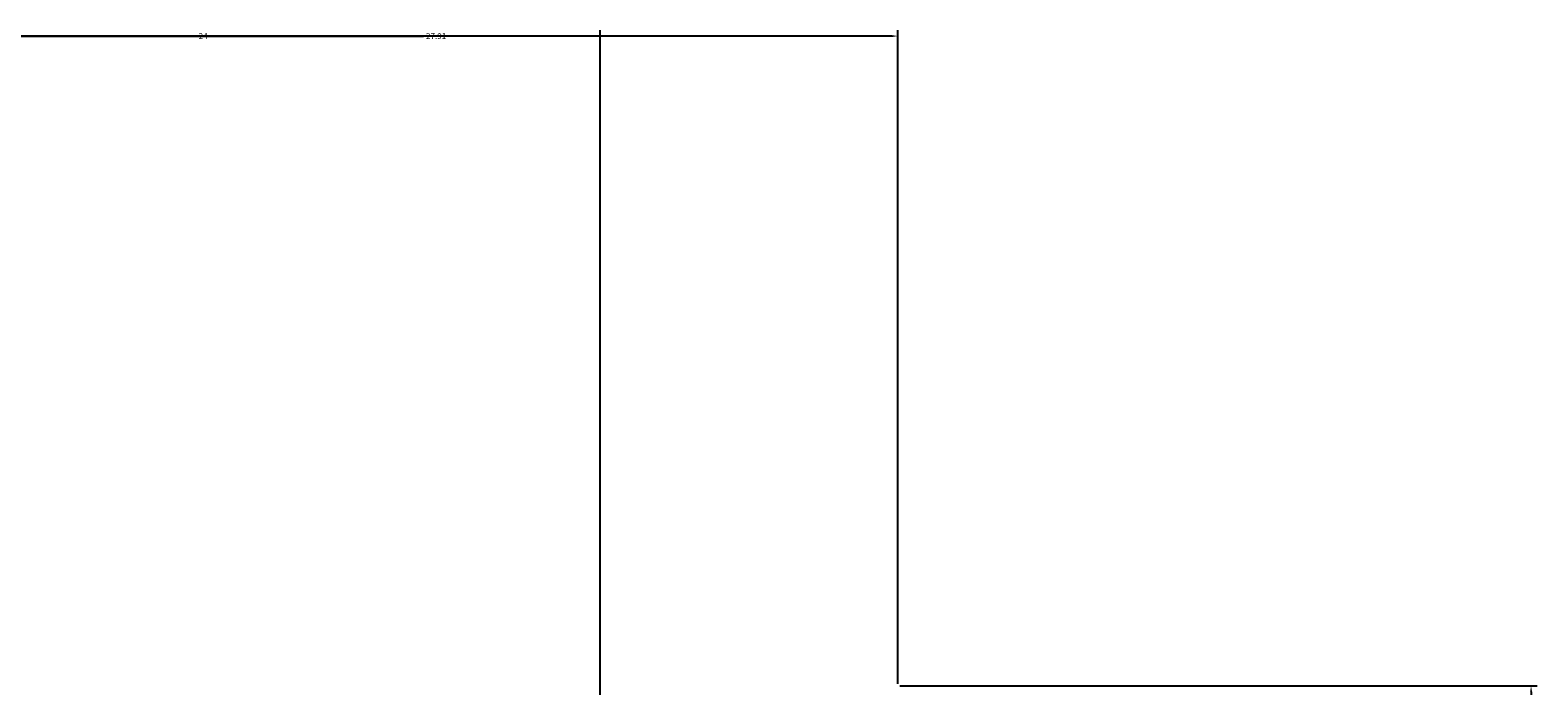
# Model space of a CAD drawing. Units: inches. Extents: x 2307 to 2544, y 2171 to 2540.
# Tile 52 of 52: x 2498 to 2544, y 2521 to 2540. Entities that reach past the tile are written whole.
import ezdxf

# ---------------------------------------------------------------- set-up
doc = ezdxf.new("R2010")
doc.units = ezdxf.units.IN
doc.layers.add('A-ANNO-DIMS', color=2, linetype='Continuous', lineweight=18)
doc.styles.get("Standard").update_dxf_attribs({"font": 'arial.ttf'})
doc.dimstyles.get("Standard").update_dxf_attribs({"dimtxt": 0.18, "dimasz": 0.18, "dimexe": 0.18, "dimexo": 0.0625, "dimgap": 0.09, "dimtad": 0, "dimtih": 1, "dimtoh": 1, "dimdec": 4, "dimzin": 0, "dimdsep": 46, "dimtxsty": 'Standard', "dimcen": 0.09, "dimadec": 0, "dimazin": 0, "dimtfac": 1, "dimtdec": 4, "dimtofl": 0, "dimtmove": 0, "dimatfit": 3, "dimfxl": 1, "dimtolj": 1, "dimtzin": 0, "dimarcsym": 0})

# ---------------------------------------------------------------- blocks, each defined once
blk = doc.blocks.new('*D37')
at = {"layer": 'A-ANNO-DIMS', "color": 0, "lineweight": -2, "transparency": 16777216}
for p, q in [((2524.758, 2520.51), (2544.026, 2520.51)), ((2543.846, 2520.33), (2543.846, 2355.692)), ((2543.846, 2190.69), (2543.846, 2355.328)), ((2524.758, 2190.51), (2544.026, 2190.51))]:
    blk.add_line(p, q, dxfattribs=at)
at = {"layer": 'A-ANNO-DIMS', "color": 0, "transparency": 16777216}
for points in [[(2543.816, 2520.33), (2543.876, 2520.33), (2543.846, 2520.51)], [(2543.816, 2190.69), (2543.876, 2190.69), (2543.846, 2190.51)]]:
    blk.add_solid(points, dxfattribs=at)
at = {"layer": 'Defpoints', "color": 0, "transparency": 16777216}
for p in [(2524.696, 2520.51), (2543.846, 2520.51), (2524.696, 2190.51)]:
    blk.add_point(p, dxfattribs=at)
at = {"layer": 'A-ANNO-DIMS', "color": 0, "transparency": 16777216, "insert": (2543.846, 2355.51), "char_height": 0.18, "attachment_point": 5}
blk.add_mtext('\\A1;330', dxfattribs=at)
blk = doc.blocks.new('*D44')
at = {"layer": 'A-ANNO-DIMS', "color": 0, "lineweight": -2, "transparency": 16777216}
for p, q in [((2496.783, 2521.077), (2496.783, 2540.345)), ((2496.963, 2540.165), (2510.362, 2540.165)), ((2524.516, 2540.165), (2511.117, 2540.165)), ((2524.696, 2520.572), (2524.696, 2540.345))]:
    blk.add_line(p, q, dxfattribs=at)
at = {"layer": 'A-ANNO-DIMS', "color": 0, "transparency": 16777216}
for points in [[(2496.963, 2540.195), (2496.963, 2540.135), (2496.783, 2540.165)], [(2524.516, 2540.195), (2524.516, 2540.135), (2524.696, 2540.165)]]:
    blk.add_solid(points, dxfattribs=at)
at = {"layer": 'Defpoints', "color": 0, "transparency": 16777216}
for p in [(2524.696, 2540.165), (2496.783, 2521.015), (2524.696, 2520.51)]:
    blk.add_point(p, dxfattribs=at)
at = {"layer": 'A-ANNO-DIMS', "color": 0, "transparency": 16777216, "insert": (2510.739, 2540.165), "char_height": 0.18, "attachment_point": 5}
blk.add_mtext('\\A1;27.91', dxfattribs=at)
blk = doc.blocks.new('*D46')
at = {"layer": 'A-ANNO-DIMS', "color": 0, "lineweight": -2, "transparency": 16777216}
for p, q in [((2455.696, 2511.572), (2455.696, 2540.345)), ((2455.876, 2540.165), (2485.477, 2540.165)), ((2515.516, 2540.165), (2485.915, 2540.165)), ((2515.696, 2511.572), (2515.696, 2540.345))]:
    blk.add_line(p, q, dxfattribs=at)
at = {"layer": 'A-ANNO-DIMS', "color": 0, "transparency": 16777216}
for points in [[(2455.876, 2540.195), (2455.876, 2540.135), (2455.696, 2540.165)], [(2515.516, 2540.195), (2515.516, 2540.135), (2515.696, 2540.165)]]:
    blk.add_solid(points, dxfattribs=at)
at = {"layer": 'Defpoints', "color": 0, "transparency": 16777216}
for p in [(2515.696, 2540.165), (2455.696, 2511.51), (2515.696, 2511.51)]:
    blk.add_point(p, dxfattribs=at)
at = {"layer": 'A-ANNO-DIMS', "color": 0, "transparency": 16777216, "insert": (2485.696, 2540.165), "char_height": 0.18, "attachment_point": 5}
blk.add_mtext('\\A1;60', dxfattribs=at)
blk = doc.blocks.new('*D61')
at = {"layer": 'A-ANNO-DIMS', "color": 0, "lineweight": -2, "transparency": 16777216}
for p, q in [((2491.696, 2435.572), (2491.696, 2540.345)), ((2491.876, 2540.165), (2503.476, 2540.165)), ((2515.516, 2540.165), (2503.916, 2540.165)), ((2515.696, 2435.572), (2515.696, 2540.345))]:
    blk.add_line(p, q, dxfattribs=at)
at = {"layer": 'A-ANNO-DIMS', "color": 0, "transparency": 16777216}
for points in [[(2491.876, 2540.195), (2491.876, 2540.135), (2491.696, 2540.165)], [(2515.516, 2540.195), (2515.516, 2540.135), (2515.696, 2540.165)]]:
    blk.add_solid(points, dxfattribs=at)
at = {"layer": 'Defpoints', "color": 0, "transparency": 16777216}
for p in [(2515.696, 2540.165), (2491.696, 2435.51), (2515.696, 2435.51)]:
    blk.add_point(p, dxfattribs=at)
at = {"layer": 'A-ANNO-DIMS', "color": 0, "transparency": 16777216, "insert": (2503.696, 2540.165), "char_height": 0.18, "attachment_point": 5}
blk.add_mtext('\\A1;24', dxfattribs=at)

msp = doc.modelspace()

# ---------------------------------------------------------------- dimensions: what is measured, and where the dimension line sits
at = {"layer": 'A-ANNO-DIMS'}
for base, p1, p2, override, picture, middle in [((2515.6958, 2540.1649), (2455.6958, 2511.5096), (2515.6958, 2511.5096), {"dimdec": 0, "dimlfac": 1, "dimrnd": 0, "dimzin": 0, "dimdsep": 46, "dimlunit": 2}, '*D46', (2485.6958, 2540.1649)), ((2515.6958, 2540.1649), (2491.6958, 2435.5096), (2515.6958, 2435.5096), {"dimdec": 0, "dimlfac": 1, "dimrnd": 0, "dimzin": 0, "dimdsep": 46, "dimlunit": 2}, '*D61', (2503.6958, 2540.1649)), ((2524.6958, 2540.1649), (2496.7832, 2521.0149), (2524.6958, 2520.5096), {"dimdec": 2, "dimlfac": 1, "dimrnd": 0, "dimzin": 0, "dimdsep": 46, "dimlunit": 2}, '*D44', (2510.7395, 2540.1649))]:
    dim = msp.add_linear_dim(base=base, p1=p1, p2=p2, dimstyle='Standard', override=override, dxfattribs=at)
    dim.commit()
    dim.dimension.update_dxf_attribs({"geometry": picture, "text_midpoint": middle})
dim = msp.add_linear_dim(base=(2543.8458, 2520.5096), p1=(2524.6958, 2190.5096), p2=(2524.6958, 2520.5096), angle=90, dimstyle='Standard', override={"dimdec": 0, "dimlfac": 1, "dimrnd": 0, "dimzin": 0, "dimdsep": 46, "dimlunit": 2}, dxfattribs=at)
dim.commit()
dim.dimension.update_dxf_attribs({"geometry": '*D37', "text_midpoint": (2543.8458, 2355.5096)})

doc.saveas('drawing.dxf')
